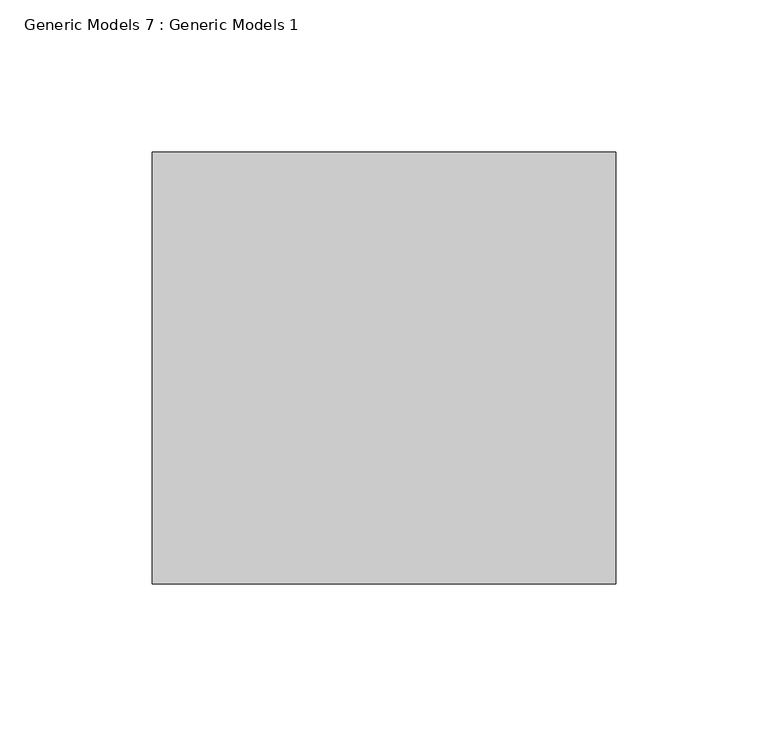
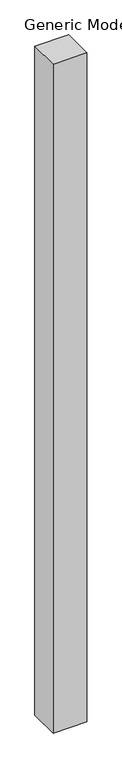
"""IFC4 building model written with IfcOpenShell, lengths in millimetres: proxy geometry, Generic Models 7 : Generic Models 1."""

from ifc_helpers import new_model, si_unit, origin, origin_with_axes, place, context, project, spatial, polyline, outline, extrude, source, transform, mapped, element, save


def generic_models_7_generic_models_1_55103d6f(model_context):
    return source(origin(), model_context, "Body", "SweptSolid", [
        extrude(outline(polyline([(-9698.5642415, -5471.7273102), (-9546.1642415, -5471.7273102), (-9546.1642415, -5613.7098142), (-9698.5642415, -5613.7098142), (-9698.5642415, -5471.7273102)])), origin_with_axes(), (0.0, 0.0, 1.0), 3200.4),
    ])


if __name__ == "__main__":
    model = new_model("IFC4")
    model_context = context("Model", 3, world=origin())
    ifc_project = project(units=[si_unit("LENGTHUNIT", "METRE", prefix="MILLI")], contexts=[model_context])
    site = spatial("IfcSite", under=ifc_project)
    building = spatial("IfcBuilding", under=site)
    placement = place(None, origin())
    generic_models_7_generic_models_1_shape = generic_models_7_generic_models_1_55103d6f(model_context)
    element("IfcBuildingElementProxy", 1, Name="Generic Models 7 : Generic Models 1", ObjectType="Generic Models 7 : Generic Models 1", at=placement, inside=building, context=model_context, shape_type="MappedRepresentation", body=[
        mapped(generic_models_7_generic_models_1_shape, transform((0.0, 0.0, 0.0), x_axis=(1.0, 0.0, 0.0), y_axis=(0.0, 1.0, 0.0), z_axis=(0.0, 0.0, 1.0))),
    ])
    save(model, "model.ifc")
